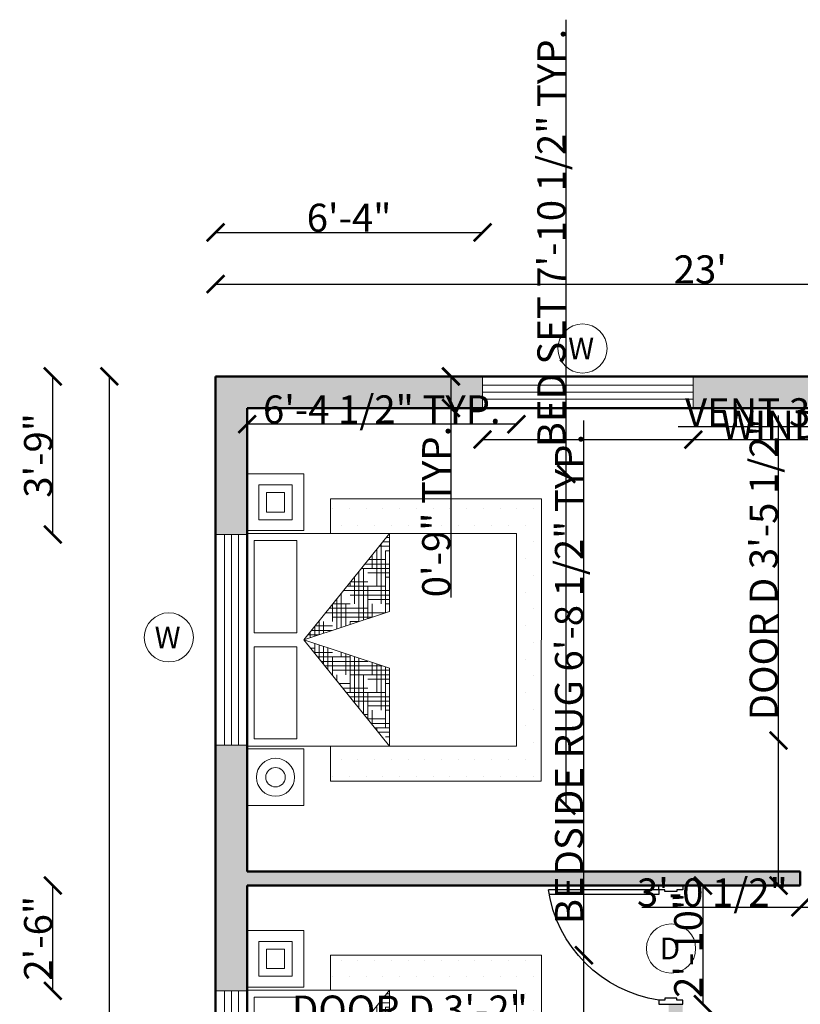
# Model space of a CAD drawing. Units: inches. Extents: x 1938 to 2373, y 1634 to 2225.
# Tile 4 of 5: x 1944 to 2167, y 1945 to 2225. Entities that reach past the tile are written whole.
import ezdxf

# ---------------------------------------------------------------- set-up
doc = ezdxf.new("R2010")
doc.units = ezdxf.units.IN
for name, color, linetype, lineweight in [('A-ANNO-DIMS', 2, 'Continuous', 18), ('A-ANNO-SYMB', 7, 'Continuous', 18), ('A-FURN', 8, 'Continuous', 18), ('A-FURN-PATT', 7, 'Continuous', 13), ('A-WALL-PATT', 82, 'Continuous', 13), ('DOOR', 30, 'Continuous', 25), ('WALL', 7, 'Continuous', 50), ('WINDOW', 150, 'Continuous', 18)]:
    doc.layers.add(name, color=color, linetype=linetype, lineweight=lineweight)
doc.styles.get("Standard").update_dxf_attribs({"font": 'arial.ttf'})
doc.dimstyles.get("Standard").update_dxf_attribs({"dimtxt": 8, "dimasz": 5, "dimexe": 0.18, "dimexo": 0.0625, "dimgap": 0.09, "dimtad": 1, "dimdec": 1, "dimzin": 0, "dimdsep": 46, "dimlunit": 4, "dimtxsty": 'Standard', "dimblk": 'ARCHTICK', "dimcen": 0.09, "dimse1": 1, "dimse2": 1, "dimadec": 0, "dimazin": 0, "dimtfac": 1, "dimtdec": 1, "dimtofl": 0, "dimtmove": 0, "dimatfit": 3, "dimfxl": 1, "dimtolj": 1, "dimtzin": 0, "dimarcsym": 0})

# ---------------------------------------------------------------- blocks, each defined once
blk = doc.blocks.new('AP0B07')
for p, q in [((33.6, 96), (33.6, 978.8)), ((72, 96), (72, 972.3)), ((0, 96), (0, -96)), ((33.6, 96), (0, 96)), ((33.6, 48), (33.6, 96)), ((48, 48), (33.6, 48)), ((48, -48), (48, 48)), ((33.6, -96), (33.6, -48)), ((33.6, -48), (48, -48)), ((0, -96), (33.6, -96))]:
    blk.add_line(p, q)
blk.add_lwpolyline([(33.6, 96), (72, 96)])
blk.add_lwpolyline([(950, 96), (950, -96), (916.4, -96), (916.4, -48), (902, -48), (902, 48), (916.4, 48), (916.4, 96)], close=True)
blk.add_arc((-123.6, -61.2), 1051.8, 8.59637, 81.40363)
blk = doc.blocks.new('*X5')
at = {"color": 0}
for p, q in [((20.25, 14.8125), (20.2772, 14.8125)), ((20.1739, 14.75), (20.2772, 14.75)), ((20.1875, 14.75), (20.1875, 14.7669)), ((20.199, 14.7812), (20.2772, 14.7812)), ((20.25, 14.3194), (20.25, 14.75)), ((20.1236, 14.6875), (20.25, 14.6875)), ((20.125, 14.5), (20.125, 14.6893)), ((20.1487, 14.7188), (20.2772, 14.7188)), ((20.1562, 14.625), (20.1562, 14.7281)), ((20.0625, 14.2573), (20.0625, 14.6116)), ((20.0938, 14.375), (20.0938, 14.6504)), ((20.0984, 14.6562), (20.125, 14.6562)), ((20.125, 14.5938), (20.2772, 14.5938)), ((20.2188, 14.3091), (20.2188, 14.625)), ((20.25, 14.625), (20.2772, 14.625)), ((19.9979, 14.5312), (20.2772, 14.5312)), ((20.023, 14.5625), (20.2772, 14.5625)), ((20.0312, 14.2469), (20.0312, 14.5727)), ((19.9476, 14.4688), (20.125, 14.4688)), ((19.9727, 14.5), (20.25, 14.5)), ((20, 14.2366), (20, 14.5)), ((20.1875, 14.2987), (20.1875, 14.5)), ((19.9062, 14.375), (19.9062, 14.4174)), ((19.9225, 14.4375), (20, 14.4375)), ((20.125, 14.4062), (20.2772, 14.4062)), ((20.25, 14.4375), (20.2772, 14.4375)), ((19.8438, 14.1848), (19.8438, 14.3397)), ((19.875, 14.25), (19.875, 14.3785)), ((19.875, 14.3438), (20.2772, 14.3438)), ((19.9688, 14.2262), (19.9688, 14.375)), ((20, 14.375), (20.2772, 14.375)), ((20.1562, 14.2884), (20.1562, 14.375)), ((19.7716, 14.25), (20, 14.25)), ((19.7812, 14.1641), (19.7812, 14.262)), ((19.7967, 14.2812), (20.125, 14.2812)), ((19.8125, 14.1744), (19.8125, 14.3008)), ((19.8219, 14.3125), (20.2291, 14.3125)), ((19.9375, 14.2159), (19.9375, 14.25)), ((19.7213, 14.1875), (19.75, 14.1875)), ((19.7465, 14.2188), (19.875, 14.2188)), ((19.75, 14.1537), (19.75, 14.2231)), ((19.7188, 14.0726), (19.7188, 14.1136)), ((19.7018, 14.0938), (19.7786, 14.0938)), ((19.7269, 14.0625), (19.8728, 14.0625)), ((19.75, 14.0338), (19.75, 14.1032)), ((19.7812, 13.9949), (19.7812, 14.0929)), ((19.8125, 14), (19.8125, 14.0825)), ((19.9062, 13.8396), (19.9062, 14.0514)), ((19.9375, 13.8007), (19.9375, 14.0411)), ((19.752, 14.0312), (19.875, 14.0312)), ((19.875, 13.8784), (19.875, 14)), ((19.875, 13.9688), (20.1557, 13.9688)), ((19.9688, 13.875), (19.9688, 14.0307)), ((20, 14), (20, 14.0204)), ((20, 14), (20.0614, 14)), ((20.0625, 13.6454), (20.0625, 13.9996)), ((20.0938, 13.625), (20.0938, 13.9893)), ((20.125, 13.75), (20.125, 13.9789)), ((20.1562, 13.875), (20.1562, 13.9686)), ((19.8275, 13.9375), (20.25, 13.9375)), ((19.8526, 13.9062), (20.125, 13.9062)), ((20.25, 13.5), (20.25, 13.9375)), ((19.8777, 13.875), (20, 13.875)), ((20.0312, 13.6842), (20.0312, 13.875)), ((20.125, 13.8438), (20.2772, 13.8438)), ((20.2188, 13.4511), (20.2188, 13.875)), ((20.25, 13.875), (20.2772, 13.875)), ((19.9532, 13.7812), (20.2772, 13.7812)), ((20, 13.8125), (20.2772, 13.8125)), ((19.9783, 13.75), (20.25, 13.75)), ((20, 13.723), (20, 13.75)), ((20.0035, 13.7188), (20.125, 13.7188)), ((20.1875, 13.49), (20.1875, 13.75)), ((20.0789, 13.625), (20.2772, 13.625)), ((20.125, 13.6562), (20.2772, 13.6562)), ((20.1562, 13.5288), (20.1562, 13.625)), ((20.25, 13.6875), (20.2772, 13.6875)), ((20.104, 13.5938), (20.2772, 13.5938)), ((20.1292, 13.5625), (20.25, 13.5625)), ((20.25, 13.5), (20.2772, 13.5)), ((20.2046, 13.4688), (20.2772, 13.4688)), ((20.2297, 13.4375), (20.2772, 13.4375)), ((20.2549, 13.4062), (20.2772, 13.4062))]:
    blk.add_line(p, q, dxfattribs=at)
blk = doc.blocks.new('MAT-P13')
for p, q in [((-1.17, 0), (-1.17, -0.4)), ((-1.17, 0), (-0.77, 0)), ((-0.77, 0), (-0.77, -0.4)), ((-0.75, 0), (0.75, 0)), ((-0.75, 0), (-0.75, -1.9)), ((0.75, 0), (0.75, -1.9)), ((0.77, 0), (1.17, 0)), ((0.77, 0), (0.77, -0.4)), ((1.17, 0), (1.17, -0.4)), ((-0.7, -0.05), (-0.7, -0.35)), ((-0.7, -0.05), (-0.05, -0.05)), ((-0.05, -0.35), (-0.05, -0.05)), ((0.05, -0.05), (0.7, -0.05)), ((0.05, -0.35), (0.05, -0.05)), ((0.7, -0.05), (0.7, -0.35)), ((-1.17, -0.4), (-0.77, -0.4)), ((-0.75, -1.0034), (0, -0.4)), ((0, -0.4), (-0.75, -1.0034)), ((-0.7, -0.35), (-0.05, -0.35)), ((0, -0.4), (-0.2, -1.0034)), ((0, -0.4), (0.2, -1.0034)), ((0, -0.4), (0.75, -1.0034)), ((0.05, -0.35), (0.7, -0.35)), ((0.77, -0.4), (1.17, -0.4)), ((-0.75, -1.0034), (-0.2, -1.0034)), ((0.2, -1.0034), (0.75, -1.0034)), ((0.75, -1.9), (-0.75, -1.9))]:
    blk.add_line(p, q)
for points in [[(0.8468, -0.0814), (1.0932, -0.0814), (1.0932, -0.3186), (0.8468, -0.3186)], [(0.9015, -0.1361), (1.0385, -0.1361), (1.0385, -0.2639), (0.9015, -0.2639)]]:
    blk.add_lwpolyline(points, close=True)
for radius in [0.1342, 0.0686]:
    blk.add_circle((-0.97, -0.2), radius)
at = {"xscale": -1, "rotation": 90}
blk.add_blockref('*X5', (14.1285, 19.2738), dxfattribs=at)
blk = doc.blocks.new('_ArchTick')
at = {"color": 0, "linetype": 'ByBlock', "const_width": 0.15}
blk.add_lwpolyline([(-0.5, -0.5), (0.5, 0.5)], dxfattribs=at)
blk = doc.blocks.new('*D12')
at = {"layer": 'A-ANNO-DIMS', "color": 0, "lineweight": -2, "transparency": 16777216}
blk.add_line((2000.23, 2149.88), (2276.23, 2149.88), dxfattribs=at)
at = {"layer": 'Defpoints', "color": 0, "transparency": 16777216}
for p in [(2276.23, 2149.88), (2000.23, 2123.59), (2276.23, 2123.59)]:
    blk.add_point(p, dxfattribs=at)
at = {"layer": 'A-ANNO-DIMS', "color": 0, "lineweight": -2, "transparency": 16777216, "xscale": 5, "yscale": 5, "zscale": 5, "rotation": 180}
blk.add_blockref('_ArchTick', (2000.23, 2149.88), dxfattribs=at)
at = {"layer": 'A-ANNO-DIMS', "color": 0, "lineweight": -2, "transparency": 16777216, "xscale": 5, "yscale": 5, "zscale": 5}
blk.add_blockref('_ArchTick', (2276.23, 2149.88), dxfattribs=at)
at = {"layer": 'A-ANNO-DIMS', "color": 0, "transparency": 16777216, "insert": (2138.23, 2154.06), "char_height": 8, "attachment_point": 5}
blk.add_mtext("\\A1;23'", dxfattribs=at)
blk = doc.blocks.new('*D13')
at = {"layer": 'A-ANNO-DIMS', "color": 0, "lineweight": -2, "transparency": 16777216}
blk.add_line((1969.98, 2123.59), (1969.98, 1667.59), dxfattribs=at)
at = {"layer": 'Defpoints', "color": 0, "transparency": 16777216}
for p in [(2000.23, 2123.59), (1969.98, 1667.59), (2000.23, 1667.59)]:
    blk.add_point(p, dxfattribs=at)
at = {"layer": 'A-ANNO-DIMS', "color": 0, "lineweight": -2, "transparency": 16777216, "xscale": 5, "yscale": 5, "zscale": 5}
for p, rotation in [((1969.98, 2123.59), 90), ((1969.98, 1667.59), 270)]:
    blk.add_blockref('_ArchTick', p, dxfattribs=dict(at, rotation=rotation))
at = {"layer": 'A-ANNO-DIMS', "color": 0, "transparency": 16777216, "insert": (1965.8, 1895.59), "char_height": 8, "attachment_point": 5, "rotation": 90}
blk.add_mtext("\\A1;38'", dxfattribs=at)
blk = doc.blocks.new('WIN-60IN')
for p, q in [((2.5, 0), (2.5, 60)), ((4.5, 0), (4.5, 60)), ((6.5, 0), (6.5, 60))]:
    blk.add_line(p, q)
blk.add_lwpolyline([(0, 0), (9, 0), (9, 60), (0, 60)], close=True)
blk = doc.blocks.new('TAG-WINDOW-W')
blk.add_circle((7, 7), 7)
blk.add_text('W', height=6.17).set_placement((2.93, 3.92))
blk = doc.blocks.new('TAG-DOOR-D')
blk.add_circle((7, 7), 7)
blk.add_text('D', height=6.17).set_placement((3.79, 3.92))
blk = doc.blocks.new('RUG-BEDSIDE')
for p, q in [((0, 70.53), (0, 80.42)), ((0, 80.42), (60.05, 80.42)), ((60, 0), (60.05, 80.42)), ((0, 10), (0, 0)), ((0, 0), (60, 0))]:
    blk.add_line(p, q)
blk = doc.blocks.new('*D21')
at = {"layer": 'A-ANNO-DIMS', "color": 0, "lineweight": -2, "transparency": 16777216}
for p, q in [((2160.51, 2019.91), (2160.51, 2112.41)), ((2160.51, 1978.59), (2160.51, 2019.91))]:
    blk.add_line(p, q, dxfattribs=at)
at = {"layer": 'Defpoints', "color": 0, "transparency": 16777216}
for p in [(2160.51, 2019.91), (2166.7, 2019.91), (2166.7, 1978.59)]:
    blk.add_point(p, dxfattribs=at)
at = {"layer": 'A-ANNO-DIMS', "color": 0, "lineweight": -2, "transparency": 16777216, "xscale": 5, "yscale": 5, "zscale": 5}
for p, rotation in [((2160.51, 2019.91), 90), ((2160.51, 1978.59), 270)]:
    blk.add_blockref('_ArchTick', p, dxfattribs=dict(at, rotation=rotation))
at = {"layer": 'A-ANNO-DIMS', "color": 0, "transparency": 16777216, "insert": (2156.27, 2068.66), "char_height": 8, "attachment_point": 5, "rotation": 90}
blk.add_mtext('\\A1;DOOR D 3\'-5 1/2"', dxfattribs=at)
blk = doc.blocks.new('*D22')
at = {"layer": 'A-ANNO-DIMS', "color": 0, "lineweight": -2, "transparency": 16777216}
for p, q in [((2166.7, 1972.39), (2121.62, 1972.39)), ((2203.23, 1972.39), (2166.7, 1972.39))]:
    blk.add_line(p, q, dxfattribs=at)
at = {"layer": 'Defpoints', "color": 0, "transparency": 16777216}
for p in [(2166.7, 1978.59), (2203.23, 1978.59), (2166.7, 1972.39)]:
    blk.add_point(p, dxfattribs=at)
at = {"layer": 'A-ANNO-DIMS', "color": 0, "lineweight": -2, "transparency": 16777216, "xscale": 5, "yscale": 5, "zscale": 5, "rotation": 180}
blk.add_blockref('_ArchTick', (2166.7, 1972.39), dxfattribs=at)
at = {"layer": 'A-ANNO-DIMS', "color": 0, "lineweight": -2, "transparency": 16777216, "xscale": 5, "yscale": 5, "zscale": 5}
blk.add_blockref('_ArchTick', (2203.23, 1972.39), dxfattribs=at)
at = {"layer": 'A-ANNO-DIMS', "color": 0, "transparency": 16777216, "insert": (2141.66, 1976.62), "char_height": 8, "attachment_point": 5}
blk.add_mtext('\\A1;3\'-0 1/2"', dxfattribs=at)
blk = doc.blocks.new('*D25')
at = {"layer": 'A-ANNO-DIMS', "color": 0, "lineweight": -2, "transparency": 16777216}
for p, q in [((2094.98, 1939.05), (2021.12, 1939.05)), ((2133.23, 1939.05), (2094.98, 1939.05))]:
    blk.add_line(p, q, dxfattribs=at)
at = {"layer": 'Defpoints', "color": 0, "transparency": 16777216}
for p in [(2094.98, 1944.79), (2133.23, 1944.79), (2094.98, 1939.05)]:
    blk.add_point(p, dxfattribs=at)
at = {"layer": 'A-ANNO-DIMS', "color": 0, "lineweight": -2, "transparency": 16777216, "xscale": 5, "yscale": 5, "zscale": 5}
for p, rotation in [((2094.98, 1939.05), 179.9999999999997), ((2133.23, 1939.05), 359.9999999999997)]:
    blk.add_blockref('_ArchTick', p, dxfattribs=dict(at, rotation=rotation))
at = {"layer": 'A-ANNO-DIMS', "color": 0, "transparency": 16777216, "insert": (2055.55, 1943.28), "char_height": 8, "attachment_point": 5}
blk.add_mtext('\\A1;DOOR D 3\'-2"', dxfattribs=at)
blk = doc.blocks.new('*D26')
at = {"layer": 'A-ANNO-DIMS', "color": 0, "lineweight": -2, "transparency": 16777216}
blk.add_line((2138.97, 1978.59), (2138.97, 1944.79), dxfattribs=at)
at = {"layer": 'Defpoints', "color": 0, "transparency": 16777216}
for p in [(2133.23, 1978.59), (2133.23, 1944.79), (2138.97, 1944.79)]:
    blk.add_point(p, dxfattribs=at)
at = {"layer": 'A-ANNO-DIMS', "color": 0, "lineweight": -2, "transparency": 16777216, "xscale": 5, "yscale": 5, "zscale": 5}
for p, rotation in [((2138.97, 1978.59), 90), ((2138.97, 1944.79), 270)]:
    blk.add_blockref('_ArchTick', p, dxfattribs=dict(at, rotation=rotation))
at = {"layer": 'A-ANNO-DIMS', "color": 0, "transparency": 16777216, "insert": (2134.79, 1961.69), "char_height": 8, "attachment_point": 5, "rotation": 90}
blk.add_mtext('\\A1;2\'-10"', dxfattribs=at)
blk = doc.blocks.new('*D29')
at = {"layer": 'A-ANNO-DIMS', "color": 0, "lineweight": -2, "transparency": 16777216}
for p, q in [((2076.23, 2105.59), (2136.23, 2105.59)), ((2136.23, 2105.59), (2256.3, 2105.59))]:
    blk.add_line(p, q, dxfattribs=at)
at = {"layer": 'Defpoints', "color": 0, "transparency": 16777216}
for p in [(2076.23, 2114.59), (2136.23, 2114.59), (2136.23, 2105.59)]:
    blk.add_point(p, dxfattribs=at)
at = {"layer": 'A-ANNO-DIMS', "color": 0, "lineweight": -2, "transparency": 16777216, "xscale": 5, "yscale": 5, "zscale": 5, "rotation": 180}
blk.add_blockref('_ArchTick', (2076.23, 2105.59), dxfattribs=at)
at = {"layer": 'A-ANNO-DIMS', "color": 0, "lineweight": -2, "transparency": 16777216, "xscale": 5, "yscale": 5, "zscale": 5}
blk.add_blockref('_ArchTick', (2136.23, 2105.59), dxfattribs=at)
at = {"layer": 'A-ANNO-DIMS', "color": 0, "transparency": 16777216, "insert": (2198.76, 2109.81), "char_height": 8, "attachment_point": 5}
blk.add_mtext('\\A1;WINDOW W 5\'-0" TYP.', dxfattribs=at)
blk = doc.blocks.new('*D30')
at = {"layer": 'A-ANNO-DIMS', "color": 0, "lineweight": -2, "transparency": 16777216}
for p, q in [((2067.23, 2123.59), (2067.23, 2114.59)), ((2067.23, 2114.59), (2067.23, 2060.64))]:
    blk.add_line(p, q, dxfattribs=at)
at = {"layer": 'Defpoints', "color": 0, "transparency": 16777216}
for p in [(2076.23, 2123.59), (2067.23, 2114.59), (2076.23, 2114.59)]:
    blk.add_point(p, dxfattribs=at)
at = {"layer": 'A-ANNO-DIMS', "color": 0, "lineweight": -2, "transparency": 16777216, "xscale": 5, "yscale": 5, "zscale": 5}
for p, rotation in [((2067.23, 2123.59), 90), ((2067.23, 2114.59), 270)]:
    blk.add_blockref('_ArchTick', p, dxfattribs=dict(at, rotation=rotation))
at = {"layer": 'A-ANNO-DIMS', "color": 0, "transparency": 16777216, "insert": (2063.05, 2085.11), "char_height": 8, "attachment_point": 5, "rotation": 90}
blk.add_mtext('\\A1;0\'-9" TYP.', dxfattribs=at)
blk = doc.blocks.new('*D35')
at = {"layer": 'A-ANNO-DIMS', "color": 0, "lineweight": -2, "transparency": 16777216}
for p, q in [((2100.06, 2095.8), (2100.06, 2225.17)), ((2100.06, 2001.37), (2100.06, 2095.8))]:
    blk.add_line(p, q, dxfattribs=at)
at = {"layer": 'Defpoints', "color": 0, "transparency": 16777216}
for p in [(2085.9, 2095.8), (2100.06, 2095.8), (2085.9, 2001.37)]:
    blk.add_point(p, dxfattribs=at)
at = {"layer": 'A-ANNO-DIMS', "color": 0, "lineweight": -2, "transparency": 16777216, "xscale": 5, "yscale": 5, "zscale": 5}
for p, rotation in [((2100.06, 2095.8), 90), ((2100.06, 2001.37), 270)]:
    blk.add_blockref('_ArchTick', p, dxfattribs=dict(at, rotation=rotation))
at = {"layer": 'A-ANNO-DIMS', "color": 0, "transparency": 16777216, "insert": (2095.84, 2162.98), "char_height": 8, "attachment_point": 5, "rotation": 90}
blk.add_mtext('\\A1;BED SET 7\'-10 1/2" TYP.', dxfattribs=at)
blk = doc.blocks.new('*D36')
at = {"layer": 'A-ANNO-DIMS', "color": 0, "lineweight": -2, "transparency": 16777216}
blk.add_line((2085.9, 2109.96), (2009.23, 2109.96), dxfattribs=at)
at = {"layer": 'Defpoints', "color": 0, "transparency": 16777216}
for p in [(2009.23, 2109.96), (2009.23, 2095.8), (2085.9, 2095.8)]:
    blk.add_point(p, dxfattribs=at)
at = {"layer": 'A-ANNO-DIMS', "color": 0, "lineweight": -2, "transparency": 16777216, "xscale": 5, "yscale": 5, "zscale": 5, "rotation": 180}
blk.add_blockref('_ArchTick', (2009.23, 2109.96), dxfattribs=at)
at = {"layer": 'A-ANNO-DIMS', "color": 0, "lineweight": -2, "transparency": 16777216, "xscale": 5, "yscale": 5, "zscale": 5}
blk.add_blockref('_ArchTick', (2085.9, 2109.96), dxfattribs=at)
at = {"layer": 'A-ANNO-DIMS', "color": 0, "transparency": 16777216, "insert": (2047.56, 2114.19), "char_height": 8, "attachment_point": 5}
blk.add_mtext('\\A1;6\'-4 1/2" TYP.', dxfattribs=at)
blk = doc.blocks.new('*D41')
at = {"layer": 'A-ANNO-DIMS', "color": 0, "lineweight": -2, "transparency": 16777216}
for p, q in [((2219.23, 2109.19), (2131.96, 2109.19)), ((2255.23, 2109.19), (2219.23, 2109.19))]:
    blk.add_line(p, q, dxfattribs=at)
at = {"layer": 'Defpoints', "color": 0, "transparency": 16777216}
for p in [(2219.23, 2114.59), (2255.23, 2114.59), (2219.23, 2109.19)]:
    blk.add_point(p, dxfattribs=at)
at = {"layer": 'A-ANNO-DIMS', "color": 0, "lineweight": -2, "transparency": 16777216, "xscale": 5, "yscale": 5, "zscale": 5}
for p, rotation in [((2219.23, 2109.19), 179.9999999999986), ((2255.23, 2109.19), 359.9999999999986)]:
    blk.add_blockref('_ArchTick', p, dxfattribs=dict(at, rotation=rotation))
at = {"layer": 'A-ANNO-DIMS', "color": 0, "transparency": 16777216, "insert": (2173.09, 2113.36), "char_height": 8, "attachment_point": 5}
blk.add_mtext('\\A1;VENT 3\'-0" TYP.', dxfattribs=at)
blk = doc.blocks.new('*D43')
at = {"layer": 'A-ANNO-DIMS', "color": 0, "lineweight": -2, "transparency": 16777216}
for p, q in [((2105.09, 1958.74), (2105.09, 2111.08)), ((2105.09, 1878.32), (2105.09, 1958.74))]:
    blk.add_line(p, q, dxfattribs=at)
at = {"layer": 'Defpoints', "color": 0, "transparency": 16777216}
for p in [(2093.02, 1958.74), (2105.09, 1958.74), (2093.02, 1878.32)]:
    blk.add_point(p, dxfattribs=at)
at = {"layer": 'A-ANNO-DIMS', "color": 0, "lineweight": -2, "transparency": 16777216, "xscale": 5, "yscale": 5, "zscale": 5}
for p, rotation in [((2105.09, 1958.74), 90), ((2105.09, 1878.32), 270)]:
    blk.add_blockref('_ArchTick', p, dxfattribs=dict(at, rotation=rotation))
at = {"layer": 'A-ANNO-DIMS', "color": 0, "transparency": 16777216, "insert": (2100.86, 2037.41), "char_height": 8, "attachment_point": 5, "rotation": 90}
blk.add_mtext('\\A1;BEDSIDE RUG 6\'-8 1/2" TYP.', dxfattribs=at)
blk = doc.blocks.new('*D58')
at = {"layer": 'A-ANNO-DIMS', "color": 0, "lineweight": -2, "transparency": 16777216}
blk.add_line((2000.23, 2164.6), (2076.23, 2164.6), dxfattribs=at)
at = {"layer": 'Defpoints', "color": 0, "transparency": 16777216}
for p in [(2076.23, 2164.6), (2000.23, 2123.59), (2076.23, 2123.59)]:
    blk.add_point(p, dxfattribs=at)
at = {"layer": 'A-ANNO-DIMS', "color": 0, "lineweight": -2, "transparency": 16777216, "xscale": 5, "yscale": 5, "zscale": 5, "rotation": 180}
blk.add_blockref('_ArchTick', (2000.23, 2164.6), dxfattribs=at)
at = {"layer": 'A-ANNO-DIMS', "color": 0, "lineweight": -2, "transparency": 16777216, "xscale": 5, "yscale": 5, "zscale": 5}
blk.add_blockref('_ArchTick', (2076.23, 2164.6), dxfattribs=at)
at = {"layer": 'A-ANNO-DIMS', "color": 0, "transparency": 16777216, "insert": (2038.23, 2168.77), "char_height": 8, "attachment_point": 5}
blk.add_mtext('\\A1;6\'-4"', dxfattribs=at)
blk = doc.blocks.new('*D60')
at = {"layer": 'A-ANNO-DIMS', "color": 0, "lineweight": -2, "transparency": 16777216}
blk.add_line((1953.9, 2078.59), (1953.9, 2123.59), dxfattribs=at)
at = {"layer": 'Defpoints', "color": 0, "transparency": 16777216}
for p in [(1953.9, 2123.59), (2000.23, 2123.59), (2000.23, 2078.59)]:
    blk.add_point(p, dxfattribs=at)
at = {"layer": 'A-ANNO-DIMS', "color": 0, "lineweight": -2, "transparency": 16777216, "xscale": 5, "yscale": 5, "zscale": 5}
for p, rotation in [((1953.9, 2123.59), 90), ((1953.9, 2078.59), 270)]:
    blk.add_blockref('_ArchTick', p, dxfattribs=dict(at, rotation=rotation))
at = {"layer": 'A-ANNO-DIMS', "color": 0, "transparency": 16777216, "insert": (1949.72, 2101.09), "char_height": 8, "attachment_point": 5, "rotation": 90}
blk.add_mtext('\\A1;3\'-9"', dxfattribs=at)
blk = doc.blocks.new('*D61')
at = {"layer": 'A-ANNO-DIMS', "color": 0, "lineweight": -2, "transparency": 16777216}
blk.add_line((1953.9, 1948.59), (1953.9, 1978.59), dxfattribs=at)
at = {"layer": 'Defpoints', "color": 0, "transparency": 16777216}
for p in [(1953.9, 1978.59), (2009.23, 1978.59), (2009.23, 1948.59)]:
    blk.add_point(p, dxfattribs=at)
at = {"layer": 'A-ANNO-DIMS', "color": 0, "lineweight": -2, "transparency": 16777216, "xscale": 5, "yscale": 5, "zscale": 5}
for p, rotation in [((1953.9, 1978.59), 90), ((1953.9, 1948.59), 270)]:
    blk.add_blockref('_ArchTick', p, dxfattribs=dict(at, rotation=rotation))
at = {"layer": 'A-ANNO-DIMS', "color": 0, "transparency": 16777216, "insert": (1949.72, 1963.59), "char_height": 8, "attachment_point": 5, "rotation": 90}
blk.add_mtext('\\A1;2\'-6"', dxfattribs=at)

msp = doc.modelspace()

# ---------------------------------------------------------------- hatches: boundary and pattern name
at = {"layer": 'A-FURN-PATT', "transparency": 33554585}
h = msp.add_hatch(dxfattribs=at)
h.set_pattern_fill('DOTS', color=256, scale=3)
h.paths.add_polyline_path([(2093.02, 2088.74), (2032.97, 2088.74), (2032.97, 2078.85), (2085.9, 2078.85), (2085.9, 2018.32), (2032.97, 2018.32), (2032.97, 2008.32), (2092.97, 2008.32)])
h.paths.add_polyline_path([(2093.02, 1958.74), (2032.97, 1958.74), (2032.97, 1948.85), (2085.9, 1948.85), (2085.9, 1888.32), (2032.97, 1888.32), (2032.97, 1878.32), (2092.97, 1878.32)])
at = {"layer": 'A-WALL-PATT', "transparency": 33554585}
h = msp.add_hatch(color=256, dxfattribs=at)
h.dxf.hatch_style = 1
h.paths.add_polyline_path([(2076.23, 2123.59), (2000.23, 2123.59), (2000.23, 2078.59), (2009.23, 2078.59), (2009.23, 2078.85), (2009.23, 2114.59), (2076.23, 2114.59)])
h.paths.add_polyline_path([(2219.23, 2123.59), (2136.23, 2123.59), (2136.23, 2114.59), (2203.23, 2114.59), (2203.23, 2085.96), (2207.23, 2085.96), (2207.23, 2114.59), (2219.23, 2114.59)])
h.paths.add_polyline_path([(2276.23, 2123.59), (2255.23, 2123.59), (2255.23, 2114.59), (2262.62, 2114.59), (2267.23, 2114.59), (2267.23, 2050.59), (2203.23, 2050.59), (2203.23, 1978.59), (2207.23, 1978.59), (2207.23, 1984.65), (2207.23, 2046.59), (2267.23, 2046.59), (2267.23, 2032.59), (2276.23, 2032.59)])
h.paths.add_polyline_path([(2009.23, 2018.59), (2000.23, 2018.59), (2000.23, 1948.59), (2009.23, 1948.59), (2009.23, 1948.85), (2009.23, 1978.59), (2126.4, 1978.59), (2126.4, 1978.59), (2133.23, 1978.59), (2166.7, 1978.59), (2166.7, 1982.59), (2009.23, 1982.59)])
h.paths.add_polyline_path([(2276.23, 1996.59), (2267.23, 1996.59), (2267.23, 1982.59), (2237.23, 1982.59), (2237.23, 1978.59), (2267.23, 1978.59), (2267.23, 1901.32), (2276.23, 1901.32)])
h.paths.add_polyline_path([(2133.23, 1944.79), (2129.23, 1944.79), (2129.23, 1858.59), (2009.23, 1858.59), (2009.23, 1888.59), (2000.23, 1888.59), (2000.23, 1839.09), (2009.23, 1839.09), (2009.23, 1854.59), (2091.31, 1854.59), (2091.31, 1854.61), (2097.36, 1854.59), (2133.23, 1854.59)])
h.paths.add_polyline_path([(2121.02, 1763.59), (2097.23, 1763.59), (2097.23, 1824.61), (2093.23, 1824.61), (2093.23, 1763.59), (2009.23, 1763.59), (2009.23, 1779.09), (2000.23, 1779.09), (2000.23, 1739.59), (2009.23, 1739.59), (2009.23, 1754.59), (2121.02, 1754.59)])
h.paths.add_polyline_path([(2108.23, 1676.59), (2009.23, 1676.59), (2009.23, 1691.59), (2000.23, 1691.59), (2000.23, 1667.59), (2108.23, 1667.59)])
h.paths.add_polyline_path([(2276.23, 1841.32), (2267.23, 1841.32), (2267.23, 1763.59), (2246.64, 1763.59), (2246.64, 1754.59), (2276.23, 1754.59)])

# ---------------------------------------------------------------- linework, layer by layer
at = {"layer": 'WALL'}
for p, q in [((2000.23, 2123.59), (2276.23, 2123.59)), ((2000.23, 2123.59), (2000.23, 1667.59)), ((2009.23, 2114.59), (2203.23, 2114.59)), ((2009.23, 2114.59), (2009.23, 1982.59)), ((2009.23, 1982.59), (2166.7, 1982.59)), ((2166.7, 1978.59), (2166.7, 1982.59)), ((2009.23, 1978.59), (2166.7, 1978.59)), ((2009.23, 1978.59), (2009.23, 1858.59))]:
    msp.add_line(p, q, dxfattribs=at)

# ---------------------------------------------------------------- block references
at = {"layer": 'A-ANNO-SYMB'}
for name, p in [('TAG-WINDOW-W', (2097.68, 2124.55)), ('TAG-WINDOW-W', (1979.95, 2042.27)), ('TAG-DOOR-D', (2122.9, 1953.67))]:
    msp.add_blockref(name, p, dxfattribs=at)
at = {"layer": 'A-FURN', "xscale": 40.35297549234498, "yscale": 40.35297549234498, "zscale": 40.35297549234498, "rotation": 90}
for p in [(2009.23, 2048.59), (2009.23, 1918.59)]:
    msp.add_blockref('MAT-P13', p, dxfattribs=at)
at = {"layer": 'A-FURN'}
for p in [(2032.97, 2008.32), (2032.97, 1878.32)]:
    msp.add_blockref('RUG-BEDSIDE', p, dxfattribs=at)
at = {"layer": 'DOOR', "xscale": -0.0355865366937081, "yscale": 0.0355865366937081, "zscale": 0.0355865366937081, "rotation": 90}
msp.add_blockref('AP0B07', (2129.81, 1978.59), dxfattribs=at)
at = {"layer": 'WINDOW', "rotation": 270.0000000000029}
msp.add_blockref('WIN-60IN', (2076.23, 2123.59), dxfattribs=at)
at = {"layer": 'WINDOW'}
for p in [(2000.23, 2018.59), (2000.23, 1888.58)]:
    msp.add_blockref('WIN-60IN', p, dxfattribs=at)

# ---------------------------------------------------------------- dimensions: what is measured, and where the dimension line sits
at = {"layer": 'A-ANNO-DIMS'}
for base, p1, p2, angle, text, picture, middle in [((2100.06, 2095.8), (2085.9, 2001.37), (2085.9, 2095.8), 90, 'BED SET <> TYP.', '*D35', (2095.84, 2162.98)), ((2136.23, 2105.59), (2076.23, 2114.59), (2136.23, 2114.59), 0, 'WINDOW W <> TYP.', '*D29', (2198.76, 2109.81)), ((2009.23, 2109.96), (2085.9, 2095.8), (2009.23, 2095.8), 180, '<> TYP.', '*D36', (2047.56, 2114.19)), ((2219.23, 2109.19), (2255.23, 2114.59), (2219.23, 2114.59), 180, 'VENT <> TYP.', '*D41', (2173.09, 2113.36)), ((2067.23, 2114.59), (2076.23, 2123.59), (2076.23, 2114.59), 270, '<> TYP.', '*D30', (2063.05, 2085.11)), ((2160.51, 2019.91), (2166.7, 1978.59), (2166.7, 2019.91), 90, 'DOOR D <>', '*D21', (2156.27, 2068.66)), ((2105.09, 1958.74), (2093.02, 1878.32), (2093.02, 1958.74), 90, 'BEDSIDE RUG <> TYP.', '*D43', (2100.86, 2037.41)), ((2094.9804, 1939.0478), (2133.2288, 1944.785), (2094.9804, 1944.785), 180, 'DOOR D <>', '*D25', (2055.5521, 1943.2796))]:
    dim = msp.add_linear_dim(base=base, p1=p1, p2=p2, angle=angle, text=text, dimstyle='Standard', override={"dimdec": 1, "dimlfac": 1, "dimrnd": 0, "dimzin": 1, "dimdsep": 46, "dimlunit": 4, "dimfrac": 2}, dxfattribs=at)
    dim.commit()
    dim.dimension.update_dxf_attribs({"geometry": picture, "text_midpoint": middle})
for base, p2, override, picture, middle in [((2076.23, 2164.6), (2076.23, 2123.59), {"dimdec": 1, "dimlfac": 1, "dimrnd": 0, "dimzin": 1, "dimdsep": 46, "dimlunit": 4, "dimfrac": 2}, '*D58', (2038.23, 2168.77)), ((2276.23, 2149.88), (2276.23, 2123.59), {"dimclrd": 0, "dimclre": 0, "dimclrt": 0}, '*D12', (2138.23, 2154.06))]:
    dim = msp.add_linear_dim(base=base, p1=(2000.23, 2123.59), p2=p2, dimstyle='Standard', override=override, dxfattribs=at)
    dim.commit()
    dim.dimension.update_dxf_attribs({"geometry": picture, "text_midpoint": middle})
for base, p1, p2, angle, override, picture, middle in [((1953.9, 2123.59), (2000.23, 2078.59), (2000.23, 2123.59), 90, {"dimdec": 1, "dimlfac": 1, "dimrnd": 0, "dimzin": 1, "dimdsep": 46, "dimlunit": 4, "dimfrac": 2}, '*D60', (1949.72, 2101.09)), ((1969.98, 1667.59), (2000.23, 2123.59), (2000.23, 1667.59), 90, {"dimclrd": 0, "dimclre": 0, "dimclrt": 0}, '*D13', (1965.8, 1895.59)), ((2166.7, 1972.39), (2203.23, 1978.59), (2166.7, 1978.59), 180, {"dimdec": 1, "dimlfac": 1, "dimrnd": 0, "dimzin": 1, "dimdsep": 46, "dimlunit": 4, "dimfrac": 2}, '*D22', (2141.66, 1976.62)), ((1953.9, 1978.59), (2009.23, 1948.59), (2009.23, 1978.59), 90, {"dimdec": 1, "dimlfac": 1, "dimrnd": 0, "dimzin": 1, "dimdsep": 46, "dimlunit": 4, "dimfrac": 2}, '*D61', (1949.72, 1963.59)), ((2138.97, 1944.79), (2133.23, 1978.59), (2133.23, 1944.79), 270, {"dimdec": 1, "dimlfac": 1, "dimrnd": 0, "dimzin": 1, "dimdsep": 46, "dimlunit": 4, "dimfrac": 2}, '*D26', (2134.79, 1961.69))]:
    dim = msp.add_linear_dim(base=base, p1=p1, p2=p2, angle=angle, dimstyle='Standard', override=override, dxfattribs=at)
    dim.commit()
    dim.dimension.update_dxf_attribs({"geometry": picture, "text_midpoint": middle})

doc.saveas('drawing.dxf')
